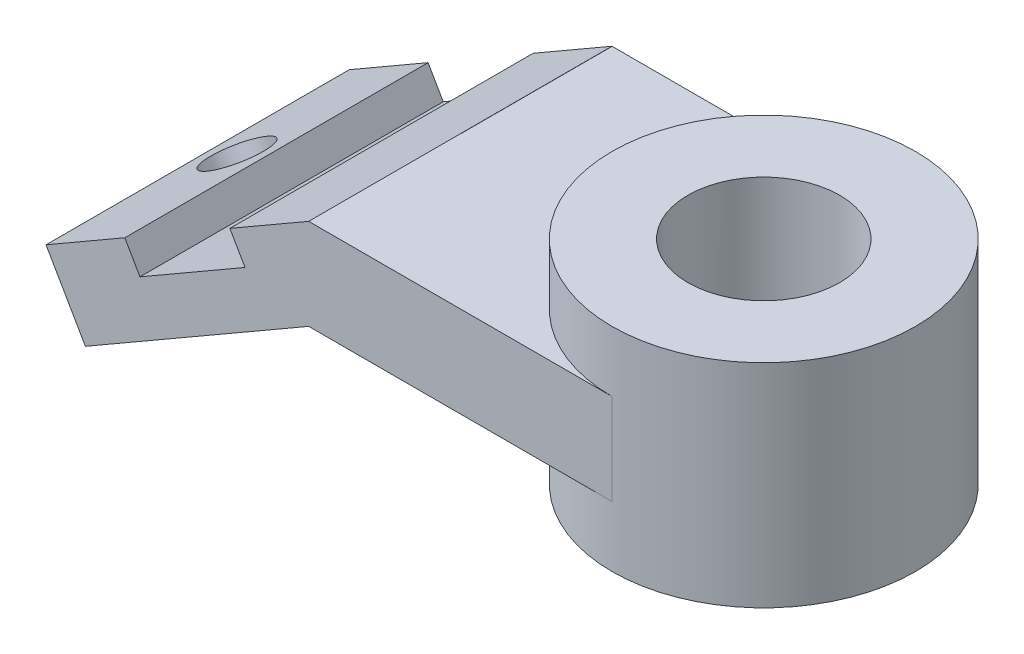
ISO-10303-21;
HEADER;
FILE_DESCRIPTION(('STEP AP214'),'2;1');
FILE_NAME('part.step','',(''),(''),'','','');
FILE_SCHEMA(('AUTOMOTIVE_DESIGN { 1 0 10303 214 1 1 1 1 }'));
ENDSEC;
DATA;
#1=APPLICATION_CONTEXT('core data for automotive mechanical design processes');
#2=APPLICATION_PROTOCOL_DEFINITION('international standard','automotive_design',2000,#1);
#3=PRODUCT_CONTEXT('',#1,'mechanical');
#4=PRODUCT('Part','Part','',(#3));
#5=PRODUCT_RELATED_PRODUCT_CATEGORY('part','',(#4));
#6=PRODUCT_DEFINITION_FORMATION('','',#4);
#7=PRODUCT_DEFINITION_CONTEXT('part definition',#1,'design');
#8=PRODUCT_DEFINITION('design','',#6,#7);
#9=PRODUCT_DEFINITION_SHAPE('','',#8);
#10=(LENGTH_UNIT() NAMED_UNIT(*) SI_UNIT(.MILLI.,.METRE.));
#11=(NAMED_UNIT(*) PLANE_ANGLE_UNIT() SI_UNIT($,.RADIAN.));
#12=(NAMED_UNIT(*) SI_UNIT($,.STERADIAN.) SOLID_ANGLE_UNIT());
#13=UNCERTAINTY_MEASURE_WITH_UNIT(LENGTH_MEASURE(1.E-05),#10,'distance_accuracy_value','');
#14=(GEOMETRIC_REPRESENTATION_CONTEXT(3) GLOBAL_UNCERTAINTY_ASSIGNED_CONTEXT((#13)) GLOBAL_UNIT_ASSIGNED_CONTEXT((#10,
#11,#12)) REPRESENTATION_CONTEXT('',''));
#15=CARTESIAN_POINT('',(0.,0.,0.));
#16=DIRECTION('',(0.,0.,1.));
#17=DIRECTION('',(1.,0.,0.));
#18=AXIS2_PLACEMENT_3D('',#15,#16,#17);
#19=CARTESIAN_POINT('',(0.,25.,25.));
#20=DIRECTION('',(0.,0.,1.));
#21=DIRECTION('',(1.,0.,0.));
#22=AXIS2_PLACEMENT_3D('',#19,#20,#21);
#23=PLANE('',#22);
#24=DIRECTION('',(-0.866025403784439,-0.5,0.));
#25=VECTOR('',#24,1.);
#26=CARTESIAN_POINT('',(-10.0071540624999,42.3328992754192,25.));
#27=LINE('',#26,#25);
#28=CARTESIAN_POINT('',(-60.5189973067666,13.1698729810777,25.));
#29=VERTEX_POINT('',#28);
#30=CARTESIAN_POINT('',(-77.8395053824553,3.16987298107774,25.));
#31=VERTEX_POINT('',#30);
#32=EDGE_CURVE('E138',#29,#31,#27,.T.);
#33=ORIENTED_EDGE('',*,*,#32,.T.);
#34=DIRECTION('',(-0.5,0.866025403784439,0.));
#35=VECTOR('',#34,1.);
#36=CARTESIAN_POINT('',(-67.8323513199554,-14.1630262943415,25.));
#37=LINE('',#36,#35);
#38=CARTESIAN_POINT('',(-80.3395053824553,7.49999999999997,25.));
#39=VERTEX_POINT('',#38);
#40=EDGE_CURVE('E148',#31,#39,#37,.T.);
#41=ORIENTED_EDGE('',*,*,#40,.T.);
#42=DIRECTION('',(-0.866025403784438,-0.500000000000001,0.));
#43=VECTOR('',#42,1.);
#44=CARTESIAN_POINT('',(-50.02861625,25.,25.));
#45=LINE('',#44,#43);
#46=CARTESIAN_POINT('',(-93.3298864392219,0.,25.));
#47=VERTEX_POINT('',#46);
#48=EDGE_CURVE('E164',#39,#47,#45,.T.);
#49=ORIENTED_EDGE('',*,*,#48,.T.);
#50=DIRECTION('',(0.500000000000002,-0.866025403784438,0.));
#51=VECTOR('',#50,1.);
#52=CARTESIAN_POINT('',(-93.3298864392219,0.,25.));
#53=LINE('',#52,#51);
#54=CARTESIAN_POINT('',(-86.8346959108386,-11.25,25.));
#55=VERTEX_POINT('',#54);
#56=EDGE_CURVE('E185',#47,#55,#53,.T.);
#57=ORIENTED_EDGE('',*,*,#56,.T.);
#58=DIRECTION('',(0.866025403784438,0.500000000000001,0.));
#59=VECTOR('',#58,1.);
#60=CARTESIAN_POINT('',(-50.02861625,10.,25.));
#61=LINE('',#60,#59);
#62=CARTESIAN_POINT('',(-50.02861625,10.,25.));
#63=VERTEX_POINT('',#62);
#64=EDGE_CURVE('E167',#55,#63,#61,.T.);
#65=ORIENTED_EDGE('',*,*,#64,.T.);
#66=DIRECTION('',(-1.,0.,0.));
#67=VECTOR('',#66,1.);
#68=CARTESIAN_POINT('',(0.,10.,25.));
#69=LINE('',#68,#67);
#70=CARTESIAN_POINT('',(0.,10.,25.));
#71=VERTEX_POINT('',#70);
#72=EDGE_CURVE('E208',#71,#63,#69,.T.);
#73=ORIENTED_EDGE('',*,*,#72,.F.);
#74=DIRECTION('',(0.,-1.,0.));
#75=VECTOR('',#74,1.);
#76=CARTESIAN_POINT('',(0.,25.,25.));
#77=LINE('',#76,#75);
#78=CARTESIAN_POINT('',(0.,25.,25.));
#79=VERTEX_POINT('',#78);
#80=EDGE_CURVE('E232',#79,#71,#77,.T.);
#81=ORIENTED_EDGE('',*,*,#80,.F.);
#82=DIRECTION('',(-1.,0.,0.));
#83=VECTOR('',#82,1.);
#84=CARTESIAN_POINT('',(0.,25.,25.));
#85=LINE('',#84,#83);
#86=CARTESIAN_POINT('',(-50.02861625,25.,25.));
#87=VERTEX_POINT('',#86);
#88=EDGE_CURVE('E228',#79,#87,#85,.T.);
#89=ORIENTED_EDGE('',*,*,#88,.T.);
#90=CARTESIAN_POINT('',(-63.0189973067666,17.5,25.));
#91=VERTEX_POINT('',#90);
#92=EDGE_CURVE('E160',#87,#91,#45,.T.);
#93=ORIENTED_EDGE('',*,*,#92,.T.);
#94=DIRECTION('',(0.5,-0.866025403784439,0.));
#95=VECTOR('',#94,1.);
#96=CARTESIAN_POINT('',(-50.5118432442666,-4.16302629434147,25.));
#97=LINE('',#96,#95);
#98=EDGE_CURVE('E147',#91,#29,#97,.T.);
#99=ORIENTED_EDGE('',*,*,#98,.T.);
#100=EDGE_LOOP('',(#33,#41,#49,#57,#65,#73,#81,#89,#93,#99));
#101=FACE_BOUND('',#100,.T.);
#102=ADVANCED_FACE('F41',(#101),#23,.T.);
#103=CARTESIAN_POINT('',(-50.02861625,25.,-25.));
#104=DIRECTION('',(-0.500000000000001,0.866025403784438,0.));
#105=DIRECTION('',(-0.866025403784438,-0.500000000000001,0.));
#106=AXIS2_PLACEMENT_3D('',#103,#104,#105);
#107=PLANE('',#106);
#108=CARTESIAN_POINT('',(-86.8346959108386,3.74999999999992,0.));
#109=DIRECTION('',(-0.500000000000001,0.866025403784438,0.));
#110=DIRECTION('',(-0.866025403784438,-0.500000000000001,0.));
#111=AXIS2_PLACEMENT_3D('',#108,#109,#110);
#112=CIRCLE('',#111,5.);
#113=CARTESIAN_POINT('',(-91.1648229297608,1.24999999999991,0.));
#114=VERTEX_POINT('',#113);
#115=EDGE_CURVE('E258',#114,#114,#112,.F.);
#116=ORIENTED_EDGE('',*,*,#115,.T.);
#117=EDGE_LOOP('',(#116));
#118=FACE_BOUND('',#117,.T.);
#119=ORIENTED_EDGE('',*,*,#48,.F.);
#120=DIRECTION('',(0.,0.,-1.));
#121=VECTOR('',#120,1.);
#122=CARTESIAN_POINT('',(-80.3395053824553,7.49999999999997,296.));
#123=LINE('',#122,#121);
#124=CARTESIAN_POINT('',(-80.3395053824553,7.49999999999997,-25.));
#125=VERTEX_POINT('',#124);
#126=EDGE_CURVE('E157',#39,#125,#123,.T.);
#127=ORIENTED_EDGE('',*,*,#126,.T.);
#128=DIRECTION('',(-0.866025403784438,-0.500000000000001,0.));
#129=VECTOR('',#128,1.);
#130=CARTESIAN_POINT('',(-50.02861625,25.,-25.));
#131=LINE('',#130,#129);
#132=CARTESIAN_POINT('',(-93.3298864392219,0.,-25.));
#133=VERTEX_POINT('',#132);
#134=EDGE_CURVE('E169',#125,#133,#131,.T.);
#135=ORIENTED_EDGE('',*,*,#134,.T.);
#136=DIRECTION('',(0.,0.,1.));
#137=VECTOR('',#136,1.);
#138=CARTESIAN_POINT('',(-93.3298864392219,0.,-25.));
#139=LINE('',#138,#137);
#140=EDGE_CURVE('E195',#133,#47,#139,.T.);
#141=ORIENTED_EDGE('',*,*,#140,.T.);
#142=EDGE_LOOP('',(#119,#127,#135,#141));
#143=FACE_BOUND('',#142,.T.);
#144=ADVANCED_FACE('F278',(#118,#143),#107,.T.);
#145=CARTESIAN_POINT('',(-50.02861625,25.,-25.));
#146=VERTEX_POINT('',#145);
#147=CARTESIAN_POINT('',(-63.0189973067666,17.5,-25.));
#148=VERTEX_POINT('',#147);
#149=EDGE_CURVE('E171',#146,#148,#131,.T.);
#150=ORIENTED_EDGE('',*,*,#149,.T.);
#151=DIRECTION('',(0.,0.,-1.));
#152=VECTOR('',#151,1.);
#153=CARTESIAN_POINT('',(-63.0189973067666,17.5,296.));
#154=LINE('',#153,#152);
#155=EDGE_CURVE('E60',#91,#148,#154,.T.);
#156=ORIENTED_EDGE('',*,*,#155,.F.);
#157=ORIENTED_EDGE('',*,*,#92,.F.);
#158=DIRECTION('',(0.,0.,1.));
#159=VECTOR('',#158,1.);
#160=CARTESIAN_POINT('',(-50.02861625,25.,0.));
#161=LINE('',#160,#159);
#162=CARTESIAN_POINT('',(-50.02861625,25.,0.));
#163=VERTEX_POINT('',#162);
#164=EDGE_CURVE('E222',#163,#87,#161,.T.);
#165=ORIENTED_EDGE('',*,*,#164,.F.);
#166=DIRECTION('',(0.,0.,1.));
#167=VECTOR('',#166,1.);
#168=CARTESIAN_POINT('',(-50.02861625,25.,-25.));
#169=LINE('',#168,#167);
#170=EDGE_CURVE('E179',#146,#163,#169,.T.);
#171=ORIENTED_EDGE('',*,*,#170,.F.);
#172=EDGE_LOOP('',(#150,#156,#157,#165,#171));
#173=FACE_BOUND('',#172,.T.);
#174=ADVANCED_FACE('F286',(#173),#107,.T.);
#175=CARTESIAN_POINT('',(0.,0.,-25.));
#176=DIRECTION('',(0.,0.,-1.));
#177=DIRECTION('',(-1.,0.,0.));
#178=AXIS2_PLACEMENT_3D('',#175,#176,#177);
#179=PLANE('',#178);
#180=ORIENTED_EDGE('',*,*,#134,.F.);
#181=DIRECTION('',(0.5,-0.866025403784439,0.));
#182=VECTOR('',#181,1.);
#183=CARTESIAN_POINT('',(-57.0070337726499,-32.9130262943415,-25.));
#184=LINE('',#183,#182);
#185=CARTESIAN_POINT('',(-77.8395053824553,3.16987298107774,-25.));
#186=VERTEX_POINT('',#185);
#187=EDGE_CURVE('E11',#125,#186,#184,.T.);
#188=ORIENTED_EDGE('',*,*,#187,.T.);
#189=DIRECTION('',(0.866025403784439,0.5,0.));
#190=VECTOR('',#189,1.);
#191=CARTESIAN_POINT('',(-20.8324716098054,36.0828992754192,-25.));
#192=LINE('',#191,#190);
#193=CARTESIAN_POINT('',(-60.5189973067666,13.1698729810777,-25.));
#194=VERTEX_POINT('',#193);
#195=EDGE_CURVE('E49',#186,#194,#192,.T.);
#196=ORIENTED_EDGE('',*,*,#195,.T.);
#197=DIRECTION('',(-0.5,0.866025403784439,0.));
#198=VECTOR('',#197,1.);
#199=CARTESIAN_POINT('',(-39.6865256969611,-22.9130262943415,-25.));
#200=LINE('',#199,#198);
#201=EDGE_CURVE('E153',#194,#148,#200,.T.);
#202=ORIENTED_EDGE('',*,*,#201,.T.);
#203=ORIENTED_EDGE('',*,*,#149,.F.);
#204=DIRECTION('',(0.,1.,0.));
#205=VECTOR('',#204,1.);
#206=CARTESIAN_POINT('',(-50.02861625,25.,-25.));
#207=LINE('',#206,#205);
#208=CARTESIAN_POINT('',(-50.02861625,10.,-25.));
#209=VERTEX_POINT('',#208);
#210=EDGE_CURVE('E168',#209,#146,#207,.T.);
#211=ORIENTED_EDGE('',*,*,#210,.F.);
#212=DIRECTION('',(0.866025403784438,0.500000000000001,0.));
#213=VECTOR('',#212,1.);
#214=CARTESIAN_POINT('',(-50.02861625,10.,-25.));
#215=LINE('',#214,#213);
#216=CARTESIAN_POINT('',(-86.8346959108386,-11.25,-25.));
#217=VERTEX_POINT('',#216);
#218=EDGE_CURVE('E180',#217,#209,#215,.T.);
#219=ORIENTED_EDGE('',*,*,#218,.F.);
#220=DIRECTION('',(0.500000000000002,-0.866025403784438,0.));
#221=VECTOR('',#220,1.);
#222=CARTESIAN_POINT('',(-93.3298864392219,0.,-25.));
#223=LINE('',#222,#221);
#224=EDGE_CURVE('E172',#133,#217,#223,.T.);
#225=ORIENTED_EDGE('',*,*,#224,.F.);
#226=EDGE_LOOP('',(#180,#188,#196,#202,#203,#211,#219,#225));
#227=FACE_BOUND('',#226,.T.);
#228=ADVANCED_FACE('F254',(#227),#179,.T.);
#229=CARTESIAN_POINT('',(0.,0.,0.));
#230=DIRECTION('',(0.,1.,0.));
#231=DIRECTION('',(0.,0.,1.));
#232=AXIS2_PLACEMENT_3D('',#229,#230,#231);
#233=CYLINDRICAL_SURFACE('',#232,25.);
#234=CARTESIAN_POINT('',(0.,35.,0.));
#235=DIRECTION('',(0.,1.,0.));
#236=DIRECTION('',(0.,0.,1.));
#237=AXIS2_PLACEMENT_3D('',#234,#235,#236);
#238=CIRCLE('',#237,25.);
#239=CARTESIAN_POINT('',(0.,35.,25.));
#240=VERTEX_POINT('',#239);
#241=EDGE_CURVE('E242',#240,#240,#238,.T.);
#242=ORIENTED_EDGE('',*,*,#241,.F.);
#243=EDGE_LOOP('',(#242));
#244=FACE_BOUND('',#243,.T.);
#245=ORIENTED_EDGE('',*,*,#80,.T.);
#246=CARTESIAN_POINT('',(0.,10.,0.));
#247=DIRECTION('',(0.,-1.,0.));
#248=DIRECTION('',(0.,0.,-1.));
#249=AXIS2_PLACEMENT_3D('',#246,#247,#248);
#250=CIRCLE('',#249,25.);
#251=CARTESIAN_POINT('',(0.,10.,-25.));
#252=VERTEX_POINT('',#251);
#253=EDGE_CURVE('E204',#71,#252,#250,.T.);
#254=ORIENTED_EDGE('',*,*,#253,.T.);
#255=DIRECTION('',(0.,-1.,0.));
#256=VECTOR('',#255,1.);
#257=CARTESIAN_POINT('',(0.,25.,-25.));
#258=LINE('',#257,#256);
#259=CARTESIAN_POINT('',(0.,25.,-25.));
#260=VERTEX_POINT('',#259);
#261=EDGE_CURVE('E231',#260,#252,#258,.T.);
#262=ORIENTED_EDGE('',*,*,#261,.F.);
#263=CARTESIAN_POINT('',(0.,25.,0.));
#264=DIRECTION('',(0.,1.,0.));
#265=DIRECTION('',(0.,0.,1.));
#266=AXIS2_PLACEMENT_3D('',#263,#264,#265);
#267=CIRCLE('',#266,25.);
#268=EDGE_CURVE('E206',#79,#260,#267,.F.);
#269=ORIENTED_EDGE('',*,*,#268,.F.);
#270=EDGE_LOOP('',(#245,#254,#262,#269));
#271=FACE_BOUND('',#270,.T.);
#272=CARTESIAN_POINT('',(0.,0.,0.));
#273=DIRECTION('',(0.,-1.,0.));
#274=DIRECTION('',(0.,0.,-1.));
#275=AXIS2_PLACEMENT_3D('',#272,#273,#274);
#276=CIRCLE('',#275,25.);
#277=CARTESIAN_POINT('',(0.,0.,-25.));
#278=VERTEX_POINT('',#277);
#279=EDGE_CURVE('E201',#278,#278,#276,.T.);
#280=ORIENTED_EDGE('',*,*,#279,.F.);
#281=EDGE_LOOP('',(#280));
#282=FACE_BOUND('',#281,.T.);
#283=ADVANCED_FACE('F43',(#244,#271,#282),#233,.T.);
#284=CARTESIAN_POINT('',(-50.,25.,0.));
#285=DIRECTION('',(-1.,0.,0.));
#286=DIRECTION('',(0.,0.,1.));
#287=AXIS2_PLACEMENT_3D('',#284,#285,#286);
#288=PLANE('',#287);
#289=DIRECTION('',(0.,-1.,0.));
#290=VECTOR('',#289,1.);
#291=CARTESIAN_POINT('',(-50.,25.,-25.));
#292=LINE('',#291,#290);
#293=CARTESIAN_POINT('',(-50.,25.,-25.));
#294=VERTEX_POINT('',#293);
#295=CARTESIAN_POINT('',(-50.,10.,-25.));
#296=VERTEX_POINT('',#295);
#297=EDGE_CURVE('E229',#294,#296,#292,.T.);
#298=ORIENTED_EDGE('',*,*,#297,.T.);
#299=DIRECTION('',(0.,0.,-1.));
#300=VECTOR('',#299,1.);
#301=CARTESIAN_POINT('',(-50.,10.,0.));
#302=LINE('',#301,#300);
#303=CARTESIAN_POINT('',(-50.,10.,0.));
#304=VERTEX_POINT('',#303);
#305=EDGE_CURVE('E62',#304,#296,#302,.T.);
#306=ORIENTED_EDGE('',*,*,#305,.F.);
#307=DIRECTION('',(0.,-1.,0.));
#308=VECTOR('',#307,1.);
#309=CARTESIAN_POINT('',(-50.,25.,0.));
#310=LINE('',#309,#308);
#311=CARTESIAN_POINT('',(-50.,25.,0.));
#312=VERTEX_POINT('',#311);
#313=EDGE_CURVE('E241',#312,#304,#310,.T.);
#314=ORIENTED_EDGE('',*,*,#313,.F.);
#315=DIRECTION('',(0.,0.,-1.));
#316=VECTOR('',#315,1.);
#317=CARTESIAN_POINT('',(-50.,25.,0.));
#318=LINE('',#317,#316);
#319=EDGE_CURVE('E218',#312,#294,#318,.T.);
#320=ORIENTED_EDGE('',*,*,#319,.T.);
#321=EDGE_LOOP('',(#298,#306,#314,#320));
#322=FACE_BOUND('',#321,.T.);
#323=ADVANCED_FACE('F294',(#322),#288,.T.);
#324=CARTESIAN_POINT('',(0.,25.,0.));
#325=DIRECTION('',(0.,0.,1.));
#326=DIRECTION('',(1.,0.,0.));
#327=AXIS2_PLACEMENT_3D('',#324,#325,#326);
#328=PLANE('',#327);
#329=DIRECTION('',(1.,0.,0.));
#330=VECTOR('',#329,1.);
#331=CARTESIAN_POINT('',(0.,10.,0.));
#332=LINE('',#331,#330);
#333=CARTESIAN_POINT('',(-50.02861625,10.,0.));
#334=VERTEX_POINT('',#333);
#335=EDGE_CURVE('E212',#334,#304,#332,.T.);
#336=ORIENTED_EDGE('',*,*,#335,.F.);
#337=DIRECTION('',(0.,-1.,0.));
#338=VECTOR('',#337,1.);
#339=CARTESIAN_POINT('',(-50.02861625,25.,0.));
#340=LINE('',#339,#338);
#341=EDGE_CURVE('E238',#163,#334,#340,.T.);
#342=ORIENTED_EDGE('',*,*,#341,.F.);
#343=DIRECTION('',(-1.,0.,0.));
#344=VECTOR('',#343,1.);
#345=CARTESIAN_POINT('',(0.,25.,0.));
#346=LINE('',#345,#344);
#347=EDGE_CURVE('E221',#312,#163,#346,.T.);
#348=ORIENTED_EDGE('',*,*,#347,.F.);
#349=ORIENTED_EDGE('',*,*,#313,.T.);
#350=EDGE_LOOP('',(#336,#342,#348,#349));
#351=FACE_BOUND('',#350,.T.);
#352=ADVANCED_FACE('F292',(#351),#328,.F.);
#353=CARTESIAN_POINT('',(0.,25.,-25.));
#354=DIRECTION('',(0.,0.,1.));
#355=DIRECTION('',(1.,0.,0.));
#356=AXIS2_PLACEMENT_3D('',#353,#354,#355);
#357=PLANE('',#356);
#358=DIRECTION('',(1.,0.,0.));
#359=VECTOR('',#358,1.);
#360=CARTESIAN_POINT('',(0.,10.,-25.));
#361=LINE('',#360,#359);
#362=EDGE_CURVE('E203',#296,#252,#361,.T.);
#363=ORIENTED_EDGE('',*,*,#362,.F.);
#364=ORIENTED_EDGE('',*,*,#297,.F.);
#365=DIRECTION('',(-1.,0.,0.));
#366=VECTOR('',#365,1.);
#367=CARTESIAN_POINT('',(0.,25.,-25.));
#368=LINE('',#367,#366);
#369=EDGE_CURVE('E226',#260,#294,#368,.T.);
#370=ORIENTED_EDGE('',*,*,#369,.F.);
#371=ORIENTED_EDGE('',*,*,#261,.T.);
#372=EDGE_LOOP('',(#363,#364,#370,#371));
#373=FACE_BOUND('',#372,.T.);
#374=ADVANCED_FACE('F289',(#373),#357,.F.);
#375=CARTESIAN_POINT('',(0.,35.,0.));
#376=DIRECTION('',(0.,1.,0.));
#377=DIRECTION('',(0.,0.,1.));
#378=AXIS2_PLACEMENT_3D('',#375,#376,#377);
#379=PLANE('',#378);
#380=CARTESIAN_POINT('',(0.,35.,0.));
#381=DIRECTION('',(0.,1.,0.));
#382=DIRECTION('',(0.,0.,1.));
#383=AXIS2_PLACEMENT_3D('',#380,#381,#382);
#384=CIRCLE('',#383,12.5);
#385=CARTESIAN_POINT('',(0.,35.,12.5));
#386=VERTEX_POINT('',#385);
#387=EDGE_CURVE('E198',#386,#386,#384,.F.);
#388=ORIENTED_EDGE('',*,*,#387,.T.);
#389=EDGE_LOOP('',(#388));
#390=FACE_BOUND('',#389,.T.);
#391=ORIENTED_EDGE('',*,*,#241,.T.);
#392=EDGE_LOOP('',(#391));
#393=FACE_BOUND('',#392,.T.);
#394=ADVANCED_FACE('F299',(#390,#393),#379,.T.);
#395=CARTESIAN_POINT('',(0.,25.,0.));
#396=DIRECTION('',(0.,1.,0.));
#397=DIRECTION('',(0.,0.,1.));
#398=AXIS2_PLACEMENT_3D('',#395,#396,#397);
#399=PLANE('',#398);
#400=ORIENTED_EDGE('',*,*,#268,.T.);
#401=ORIENTED_EDGE('',*,*,#369,.T.);
#402=ORIENTED_EDGE('',*,*,#319,.F.);
#403=ORIENTED_EDGE('',*,*,#347,.T.);
#404=ORIENTED_EDGE('',*,*,#164,.T.);
#405=ORIENTED_EDGE('',*,*,#88,.F.);
#406=EDGE_LOOP('',(#400,#401,#402,#403,#404,#405));
#407=FACE_BOUND('',#406,.T.);
#408=ADVANCED_FACE('F301',(#407),#399,.T.);
#409=CARTESIAN_POINT('',(0.,10.,0.));
#410=DIRECTION('',(0.,-1.,0.));
#411=DIRECTION('',(0.,0.,-1.));
#412=AXIS2_PLACEMENT_3D('',#409,#410,#411);
#413=PLANE('',#412);
#414=ORIENTED_EDGE('',*,*,#253,.F.);
#415=ORIENTED_EDGE('',*,*,#72,.T.);
#416=DIRECTION('',(0.,0.,-1.));
#417=VECTOR('',#416,1.);
#418=CARTESIAN_POINT('',(-50.02861625,10.,0.));
#419=LINE('',#418,#417);
#420=EDGE_CURVE('E211',#63,#334,#419,.T.);
#421=ORIENTED_EDGE('',*,*,#420,.T.);
#422=ORIENTED_EDGE('',*,*,#335,.T.);
#423=ORIENTED_EDGE('',*,*,#305,.T.);
#424=ORIENTED_EDGE('',*,*,#362,.T.);
#425=EDGE_LOOP('',(#414,#415,#421,#422,#423,#424));
#426=FACE_BOUND('',#425,.T.);
#427=ADVANCED_FACE('F308',(#426),#413,.T.);
#428=CARTESIAN_POINT('',(0.,0.,0.));
#429=DIRECTION('',(0.,-1.,0.));
#430=DIRECTION('',(0.,0.,-1.));
#431=AXIS2_PLACEMENT_3D('',#428,#429,#430);
#432=PLANE('',#431);
#433=CARTESIAN_POINT('',(0.,0.,0.));
#434=DIRECTION('',(0.,-1.,0.));
#435=DIRECTION('',(0.,0.,-1.));
#436=AXIS2_PLACEMENT_3D('',#433,#434,#435);
#437=CIRCLE('',#436,12.5);
#438=CARTESIAN_POINT('',(0.,0.,-12.5));
#439=VERTEX_POINT('',#438);
#440=EDGE_CURVE('E188',#439,#439,#437,.F.);
#441=ORIENTED_EDGE('',*,*,#440,.T.);
#442=EDGE_LOOP('',(#441));
#443=FACE_BOUND('',#442,.T.);
#444=ORIENTED_EDGE('',*,*,#279,.T.);
#445=EDGE_LOOP('',(#444));
#446=FACE_BOUND('',#445,.T.);
#447=ADVANCED_FACE('F324',(#443,#446),#432,.T.);
#448=CARTESIAN_POINT('',(0.,69.,0.));
#449=DIRECTION('',(0.,-1.,0.));
#450=DIRECTION('',(0.,0.,-1.));
#451=AXIS2_PLACEMENT_3D('',#448,#449,#450);
#452=CYLINDRICAL_SURFACE('',#451,12.5);
#453=ORIENTED_EDGE('',*,*,#387,.F.);
#454=EDGE_LOOP('',(#453));
#455=FACE_BOUND('',#454,.T.);
#456=ORIENTED_EDGE('',*,*,#440,.F.);
#457=EDGE_LOOP('',(#456));
#458=FACE_BOUND('',#457,.T.);
#459=ADVANCED_FACE('F321',(#455,#458),#452,.F.);
#460=CARTESIAN_POINT('',(-50.02861625,25.,-25.));
#461=DIRECTION('',(1.,0.,0.));
#462=DIRECTION('',(0.,0.,-1.));
#463=AXIS2_PLACEMENT_3D('',#460,#461,#462);
#464=PLANE('',#463);
#465=ORIENTED_EDGE('',*,*,#170,.T.);
#466=ORIENTED_EDGE('',*,*,#341,.T.);
#467=DIRECTION('',(0.,0.,1.));
#468=VECTOR('',#467,1.);
#469=CARTESIAN_POINT('',(-50.02861625,10.,-25.));
#470=LINE('',#469,#468);
#471=EDGE_CURVE('E190',#209,#334,#470,.T.);
#472=ORIENTED_EDGE('',*,*,#471,.F.);
#473=ORIENTED_EDGE('',*,*,#210,.T.);
#474=EDGE_LOOP('',(#465,#466,#472,#473));
#475=FACE_BOUND('',#474,.T.);
#476=ADVANCED_FACE('F328',(#475),#464,.T.);
#477=CARTESIAN_POINT('',(-50.02861625,10.,-25.));
#478=DIRECTION('',(0.500000000000001,-0.866025403784438,0.));
#479=DIRECTION('',(0.866025403784438,0.500000000000001,0.));
#480=AXIS2_PLACEMENT_3D('',#477,#478,#479);
#481=PLANE('',#480);
#482=CARTESIAN_POINT('',(-80.3395053824553,-7.50000000000006,0.));
#483=DIRECTION('',(0.500000000000001,-0.866025403784438,0.));
#484=DIRECTION('',(0.866025403784438,0.500000000000001,0.));
#485=AXIS2_PLACEMENT_3D('',#482,#483,#484);
#486=CIRCLE('',#485,5.);
#487=CARTESIAN_POINT('',(-76.0093783635331,-5.00000000000006,0.));
#488=VERTEX_POINT('',#487);
#489=EDGE_CURVE('E44',#488,#488,#486,.F.);
#490=ORIENTED_EDGE('',*,*,#489,.T.);
#491=EDGE_LOOP('',(#490));
#492=FACE_BOUND('',#491,.T.);
#493=ORIENTED_EDGE('',*,*,#64,.F.);
#494=DIRECTION('',(0.,0.,1.));
#495=VECTOR('',#494,1.);
#496=CARTESIAN_POINT('',(-86.8346959108386,-11.25,-25.));
#497=LINE('',#496,#495);
#498=EDGE_CURVE('E194',#217,#55,#497,.T.);
#499=ORIENTED_EDGE('',*,*,#498,.F.);
#500=ORIENTED_EDGE('',*,*,#218,.T.);
#501=ORIENTED_EDGE('',*,*,#471,.T.);
#502=ORIENTED_EDGE('',*,*,#420,.F.);
#503=EDGE_LOOP('',(#493,#499,#500,#501,#502));
#504=FACE_BOUND('',#503,.T.);
#505=ADVANCED_FACE('F266',(#492,#504),#481,.T.);
#506=CARTESIAN_POINT('',(-93.3298864392219,0.,-25.));
#507=DIRECTION('',(-0.866025403784438,-0.500000000000002,0.));
#508=DIRECTION('',(0.500000000000002,-0.866025403784438,0.));
#509=AXIS2_PLACEMENT_3D('',#506,#507,#508);
#510=PLANE('',#509);
#511=ORIENTED_EDGE('',*,*,#56,.F.);
#512=ORIENTED_EDGE('',*,*,#140,.F.);
#513=ORIENTED_EDGE('',*,*,#224,.T.);
#514=ORIENTED_EDGE('',*,*,#498,.T.);
#515=EDGE_LOOP('',(#511,#512,#513,#514));
#516=FACE_BOUND('',#515,.T.);
#517=ADVANCED_FACE('F340',(#516),#510,.T.);
#518=CARTESIAN_POINT('',(-80.3395053824553,7.49999999999997,296.));
#519=DIRECTION('',(0.866025403784439,0.5,0.));
#520=DIRECTION('',(-0.5,0.866025403784439,0.));
#521=AXIS2_PLACEMENT_3D('',#518,#519,#520);
#522=PLANE('',#521);
#523=DIRECTION('',(0.,0.,-1.));
#524=VECTOR('',#523,1.);
#525=CARTESIAN_POINT('',(-77.8395053824553,3.16987298107774,296.));
#526=LINE('',#525,#524);
#527=EDGE_CURVE('E143',#31,#186,#526,.T.);
#528=ORIENTED_EDGE('',*,*,#527,.T.);
#529=ORIENTED_EDGE('',*,*,#187,.F.);
#530=ORIENTED_EDGE('',*,*,#126,.F.);
#531=ORIENTED_EDGE('',*,*,#40,.F.);
#532=EDGE_LOOP('',(#528,#529,#530,#531));
#533=FACE_BOUND('',#532,.T.);
#534=ADVANCED_FACE('F259',(#533),#522,.T.);
#535=CARTESIAN_POINT('',(-77.8395053824553,3.16987298107774,296.));
#536=DIRECTION('',(-0.5,0.866025403784439,0.));
#537=DIRECTION('',(-0.866025403784439,-0.5,0.));
#538=AXIS2_PLACEMENT_3D('',#535,#536,#537);
#539=PLANE('',#538);
#540=DIRECTION('',(0.,0.,-1.));
#541=VECTOR('',#540,1.);
#542=CARTESIAN_POINT('',(-60.5189973067666,13.1698729810777,296.));
#543=LINE('',#542,#541);
#544=EDGE_CURVE('E145',#29,#194,#543,.T.);
#545=ORIENTED_EDGE('',*,*,#544,.T.);
#546=ORIENTED_EDGE('',*,*,#195,.F.);
#547=ORIENTED_EDGE('',*,*,#527,.F.);
#548=ORIENTED_EDGE('',*,*,#32,.F.);
#549=EDGE_LOOP('',(#545,#546,#547,#548));
#550=FACE_BOUND('',#549,.T.);
#551=ADVANCED_FACE('F142',(#550),#539,.T.);
#552=CARTESIAN_POINT('',(-63.0189973067666,17.5,296.));
#553=DIRECTION('',(-0.866025403784439,-0.499999999999999,0.));
#554=DIRECTION('',(0.5,-0.866025403784439,0.));
#555=AXIS2_PLACEMENT_3D('',#552,#553,#554);
#556=PLANE('',#555);
#557=ORIENTED_EDGE('',*,*,#155,.T.);
#558=ORIENTED_EDGE('',*,*,#201,.F.);
#559=ORIENTED_EDGE('',*,*,#544,.F.);
#560=ORIENTED_EDGE('',*,*,#98,.F.);
#561=EDGE_LOOP('',(#557,#558,#559,#560));
#562=FACE_BOUND('',#561,.T.);
#563=ADVANCED_FACE('F155',(#562),#556,.T.);
#564=CARTESIAN_POINT('',(-176.334695910839,158.768547277414,0.));
#565=DIRECTION('',(0.500000000000001,-0.866025403784438,0.));
#566=DIRECTION('',(0.866025403784438,0.500000000000001,0.));
#567=AXIS2_PLACEMENT_3D('',#564,#565,#566);
#568=CYLINDRICAL_SURFACE('',#567,5.);
#569=ORIENTED_EDGE('',*,*,#115,.F.);
#570=EDGE_LOOP('',(#569));
#571=FACE_BOUND('',#570,.T.);
#572=ORIENTED_EDGE('',*,*,#489,.F.);
#573=EDGE_LOOP('',(#572));
#574=FACE_BOUND('',#573,.T.);
#575=ADVANCED_FACE('F268',(#571,#574),#568,.F.);
#576=CLOSED_SHELL('',(#102,#144,#174,#228,#283,#323,#352,#374,#394,#408,#427,#447,#459,#476,
#505,#517,#534,#551,#563,#575));
#577=MANIFOLD_SOLID_BREP('B2',#576);
#578=ADVANCED_BREP_SHAPE_REPRESENTATION('',(#18,#577),#14);
#579=SHAPE_DEFINITION_REPRESENTATION(#9,#578);
ENDSEC;
END-ISO-10303-21;
